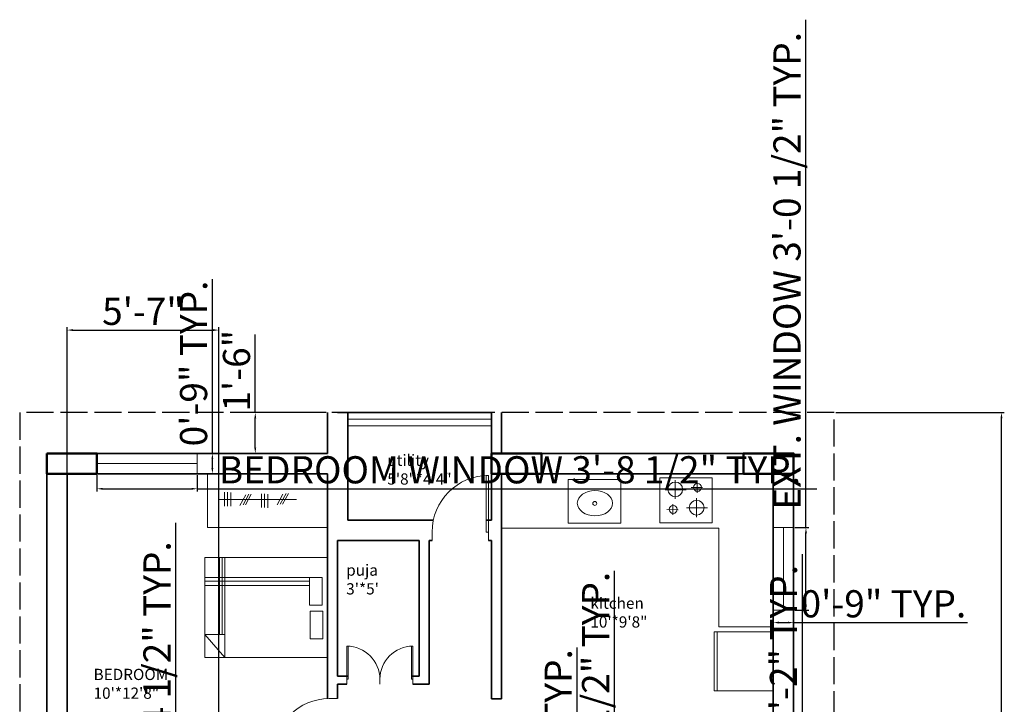
# Model space of a CAD drawing. Units: inches. Extents: x 2147 to 2722, y 2048 to 2905.
# Tile 3 of 3: x 2209 to 2644, y 2602 to 2905. Entities that reach past the tile are written whole.
import ezdxf

# ---------------------------------------------------------------- set-up
doc = ezdxf.new("R2010")
doc.units = ezdxf.units.IN
doc.linetypes.add('ACAD_ISO02W100', pattern=[15, 12, -3])
for name, color, linetype, lineweight in [('A-ANNO-DIMS', 2, 'Continuous', 18), ('A-AREA-IDEN', 7, 'Continuous', 18), ('A-COLS', 7, 'Continuous', 50), ('A-COLS-PATT', 252, 'Continuous', 13), ('A-DOOR', 3, 'Continuous', 18), ('A-EQPM', 9, 'Continuous', 18), ('A-FLOR-CASE', 8, 'Continuous', 18), ('A-FLOR-FIXT', 9, 'Continuous', 18), ('A-FURN', 8, 'Continuous', 18), ('A-GLAZ', 4, 'Continuous', 18), ('A-WALL', 7, 'Continuous', 35), ('C-PROP', 6, 'ACAD_ISO02W100', 25)]:
    doc.layers.add(name, color=color, linetype=linetype, lineweight=lineweight)
doc.styles.get("Standard").update_dxf_attribs({"font": 'arial.ttf'})
doc.dimstyles.new('ISO-25', dxfattribs={"dimtxt": 12, "dimasz": 2.5, "dimexe": 1.25, "dimexo": 0.625, "dimtad": 1, "dimdec": 0, "dimlunit": 4, "dimtxsty": 'Standard', "dimcen": 2.5, "dimadec": 0, "dimazin": 0, "dimtfac": 1, "dimtdec": 0, "dimtmove": 0, "dimatfit": 3, "dimfxl": 1, "dimarcsym": 0})

# ---------------------------------------------------------------- blocks, each defined once
blk = doc.blocks.new('*D1')
at = {"layer": 'A-ANNO-DIMS', "color": 0, "lineweight": -2, "transparency": 16777216}
for p, q in [((2569.22, 2730.99), (2643.73, 2730.99)), ((2642.48, 2133.49), (2642.48, 2728.49)), ((2569.22, 2130.99), (2643.73, 2130.99))]:
    blk.add_line(p, q, dxfattribs=at)
at = {"layer": 'A-ANNO-DIMS', "color": 0, "lineweight": 100, "transparency": 16777216}
for points in [[(2642.06, 2728.49), (2642.9, 2728.49), (2642.48, 2730.99)], [(2642.06, 2133.49), (2642.9, 2133.49), (2642.48, 2130.99)]]:
    blk.add_solid(points, dxfattribs=at)
at = {"layer": 'Defpoints', "color": 0, "lineweight": 100, "transparency": 16777216}
for p in [(2568.6, 2730.99), (2642.48, 2730.99), (2568.6, 2130.99)]:
    blk.add_point(p, dxfattribs=at)
at = {"layer": 'A-ANNO-DIMS', "color": 0, "transparency": 16777216, "insert": (2635.73, 2430.99), "char_height": 12, "attachment_point": 5, "rotation": 90}
blk.add_mtext("50'", dxfattribs=at)
blk = doc.blocks.new('*U3')
for p, q in [((0, 0), (0, -6)), ((40, 0), (40, -6))]:
    blk.add_line(p, q)
blk.add_lwpolyline([(0, 0), (0, 40), (1.75, 40), (1.75, 0)], close=True)
blk.add_arc((0, 0), 40, 0, 90)
blk = doc.blocks.new('*D7')
at = {"layer": 'A-ANNO-DIMS', "color": 0, "lineweight": -2, "transparency": 16777216}
for p, q in [((2312.71, 2730.99), (2312.71, 2765.51)), ((2343.97, 2730.99), (2311.46, 2730.99)), ((2312.71, 2715.49), (2312.71, 2728.49)), ((2343.97, 2712.99), (2311.46, 2712.99))]:
    blk.add_line(p, q, dxfattribs=at)
at = {"layer": 'A-ANNO-DIMS', "color": 0, "lineweight": 100, "transparency": 16777216}
for points in [[(2312.29, 2728.49), (2313.13, 2728.49), (2312.71, 2730.99)], [(2312.29, 2715.49), (2313.13, 2715.49), (2312.71, 2712.99)]]:
    blk.add_solid(points, dxfattribs=at)
at = {"layer": 'Defpoints', "color": 0, "lineweight": 100, "transparency": 16777216}
for p in [(2312.71, 2730.99), (2344.59, 2730.99), (2344.59, 2712.99)]:
    blk.add_point(p, dxfattribs=at)
at = {"layer": 'A-ANNO-DIMS', "color": 0, "transparency": 16777216, "insert": (2305.96, 2749.5), "char_height": 12, "attachment_point": 5, "rotation": 90}
blk.add_mtext('1\'-6"', dxfattribs=at)
blk = doc.blocks.new('BED-TWIN-PILLOW')
for p, q in [((6.6, 10.17), (6.6, 44.18)), ((7.66, 10.17), (7.66, 44.18)), ((8.88, 10.17), (8.88, 44.18)), ((46.28, 35.34), (0, 35.34)), ((46.28, 33.66), (0, 33.66)), ((46.28, 31.83), (0, 31.83)), ((8.88, 0), (0, 10.17))]:
    blk.add_line(p, q)
for points in [[(54.22, 44.18), (0, 44.18), (0, 0), (54.22, 0)], [(51.93, 35.34), (46.28, 35.34), (46.28, 23.14), (51.93, 23.14)], [(52.24, 20.39), (46.59, 20.39), (46.59, 8.19), (52.24, 8.19)], [(0, 0), (8.88, 0), (8.88, 10.17), (0, 10.17)]]:
    blk.add_lwpolyline(points, close=True)
blk = doc.blocks.new('WARDROBE')
for p, q in [((7.59, 9.5), (7.59, 15.59)), ((8.92, 9.5), (8.92, 15.59)), ((10.35, 9.4), (10.35, 15.5)), ((14.36, 9.78), (16.93, 14.55)), ((15.74, 10.07), (18.32, 14.83)), ((16.79, 10.07), (19.36, 14.83)), ((23.89, 8.83), (23.89, 14.93)), ((25.23, 8.83), (25.23, 14.93)), ((26.66, 8.73), (26.66, 14.83)), ((30.8, 10.05), (33.37, 14.82)), ((32.18, 10.34), (34.76, 15.1)), ((33.23, 10.34), (35.81, 15.1)), ((5.01, 12.45), (39.39, 12.45))]:
    blk.add_line(p, q)
blk.add_lwpolyline([(53.03, 23.8), (0, 23.8), (0, 0), (53.03, 0)], close=True)
blk = doc.blocks.new('WINDOW-BEDROOM')
blk.add_line((0, 4.5), (44.35, 4.5))
blk.add_lwpolyline([(0, 9), (44.35, 9), (44.35, 0), (0, 0)], close=True)
blk = doc.blocks.new('WINDOW-EXTERIOR')
blk.add_line((4.5, 36.51), (4.5, 0))
blk.add_lwpolyline([(0, 36.51), (9, 36.51), (9, 0), (0, 0)], close=True)
blk = doc.blocks.new('*D25')
at = {"layer": 'A-ANNO-DIMS', "color": 0, "lineweight": -2, "transparency": 16777216}
for p, q in [((2471.49, 2556.24), (2471.49, 2661.1)), ((2470.57, 2556.24), (2472.74, 2556.24)), ((2471.49, 2549.26), (2471.49, 2553.74)), ((2470.57, 2546.76), (2472.74, 2546.76))]:
    blk.add_line(p, q, dxfattribs=at)
at = {"layer": 'A-ANNO-DIMS', "color": 0, "lineweight": 100, "transparency": 16777216}
for points in [[(2471.08, 2553.74), (2471.91, 2553.74), (2471.49, 2556.24)], [(2471.08, 2549.26), (2471.91, 2549.26), (2471.49, 2546.76)]]:
    blk.add_solid(points, dxfattribs=at)
at = {"layer": 'Defpoints', "color": 0, "lineweight": 100, "transparency": 16777216}
for p in [(2469.94, 2556.24), (2471.49, 2556.24), (2469.94, 2546.76)]:
    blk.add_point(p, dxfattribs=at)
at = {"layer": 'A-ANNO-DIMS', "color": 0, "transparency": 16777216, "insert": (2464.66, 2609.92), "char_height": 12, "attachment_point": 5, "rotation": 90}
blk.add_mtext('0\'-9 1/2" TYP.', dxfattribs=at)
blk = doc.blocks.new('*D32')
at = {"layer": 'A-ANNO-DIMS', "color": 0, "lineweight": -2, "transparency": 16777216}
for p, q in [((2556.07, 2680.2), (2556.07, 2904.56)), ((2551.22, 2680.2), (2557.32, 2680.2)), ((2556.07, 2646.2), (2556.07, 2677.7)), ((2551.22, 2643.7), (2557.32, 2643.7))]:
    blk.add_line(p, q, dxfattribs=at)
at = {"layer": 'A-ANNO-DIMS', "color": 0, "lineweight": 100, "transparency": 16777216}
for points in [[(2555.66, 2677.7), (2556.49, 2677.7), (2556.07, 2680.2)], [(2555.66, 2646.2), (2556.49, 2646.2), (2556.07, 2643.7)]]:
    blk.add_solid(points, dxfattribs=at)
at = {"layer": 'Defpoints', "color": 0, "lineweight": 100, "transparency": 16777216}
for p in [(2550.6, 2680.2), (2556.07, 2680.2), (2550.6, 2643.7)]:
    blk.add_point(p, dxfattribs=at)
at = {"layer": 'A-ANNO-DIMS', "color": 0, "transparency": 16777216, "insert": (2549.24, 2793.63), "char_height": 12, "attachment_point": 5, "rotation": 90}
blk.add_mtext('EXT. WINDOW 3\'-0 1/2" TYP.', dxfattribs=at)
blk = doc.blocks.new('*D33')
at = {"layer": 'A-ANNO-DIMS', "color": 0, "lineweight": -2, "transparency": 16777216}
for p, q in [((2541.6, 2643.07), (2541.6, 2636.97)), ((2550.6, 2643.07), (2550.6, 2636.97)), ((2544.1, 2638.22), (2548.1, 2638.22)), ((2550.6, 2638.22), (2627.49, 2638.22))]:
    blk.add_line(p, q, dxfattribs=at)
at = {"layer": 'A-ANNO-DIMS', "color": 0, "lineweight": 100, "transparency": 16777216}
for points in [[(2544.1, 2638.64), (2544.1, 2637.81), (2541.6, 2638.22)], [(2548.1, 2638.64), (2548.1, 2637.81), (2550.6, 2638.22)]]:
    blk.add_solid(points, dxfattribs=at)
at = {"layer": 'Defpoints', "color": 0, "lineweight": 100, "transparency": 16777216}
for p in [(2541.6, 2643.7), (2550.6, 2643.7), (2550.6, 2638.22)]:
    blk.add_point(p, dxfattribs=at)
at = {"layer": 'A-ANNO-DIMS', "color": 0, "transparency": 16777216, "insert": (2590.3, 2644.97), "char_height": 12, "attachment_point": 5}
blk.add_mtext('0\'-9" TYP.', dxfattribs=at)
blk = doc.blocks.new('*D37')
at = {"layer": 'A-ANNO-DIMS', "color": 0, "lineweight": -2, "transparency": 16777216}
for p, q in [((2454.9, 2540.96), (2454.9, 2627.18)), ((2453.83, 2540.96), (2456.15, 2540.96)), ((2454.9, 2532.23), (2454.9, 2538.46)), ((2453.83, 2529.73), (2456.15, 2529.73))]:
    blk.add_line(p, q, dxfattribs=at)
at = {"layer": 'A-ANNO-DIMS', "color": 0, "lineweight": 100, "transparency": 16777216}
for points in [[(2454.48, 2538.46), (2455.32, 2538.46), (2454.9, 2540.96)], [(2454.48, 2532.23), (2455.32, 2532.23), (2454.9, 2529.73)]]:
    blk.add_solid(points, dxfattribs=at)
at = {"layer": 'Defpoints', "color": 0, "lineweight": 100, "transparency": 16777216}
for p in [(2453.21, 2540.96), (2454.9, 2540.96), (2453.21, 2529.73)]:
    blk.add_point(p, dxfattribs=at)
at = {"layer": 'A-ANNO-DIMS', "color": 0, "transparency": 16777216, "insert": (2448.15, 2585.32), "char_height": 12, "attachment_point": 5, "rotation": 90}
blk.add_mtext('0\'-11" TYP.', dxfattribs=at)
blk = doc.blocks.new('*D40')
at = {"layer": 'A-ANNO-DIMS', "color": 0, "lineweight": -2, "transparency": 16777216}
for p, q in [((2242.74, 2703.36), (2242.74, 2696.09)), ((2287.1, 2703.36), (2287.1, 2696.09)), ((2245.24, 2697.34), (2284.6, 2697.34)), ((2287.1, 2697.34), (2560.91, 2697.34))]:
    blk.add_line(p, q, dxfattribs=at)
at = {"layer": 'A-ANNO-DIMS', "color": 0, "lineweight": 100, "transparency": 16777216}
for points in [[(2245.24, 2697.75), (2245.24, 2696.92), (2242.74, 2697.34)], [(2284.6, 2697.75), (2284.6, 2696.92), (2287.1, 2697.34)]]:
    blk.add_solid(points, dxfattribs=at)
at = {"layer": 'Defpoints', "color": 0, "lineweight": 100, "transparency": 16777216}
for p in [(2242.74, 2703.99), (2287.1, 2703.99), (2287.1, 2697.34)]:
    blk.add_point(p, dxfattribs=at)
at = {"layer": 'A-ANNO-DIMS', "color": 0, "transparency": 16777216, "insert": (2425.25, 2704.17), "char_height": 12, "attachment_point": 5}
blk.add_mtext('BEDROOM WINDOW 3\'-8 1/2" TYP.', dxfattribs=at)
blk = doc.blocks.new('*D41')
at = {"layer": 'A-ANNO-DIMS', "color": 0, "lineweight": -2, "transparency": 16777216}
for p, q in [((2293.75, 2712.99), (2293.75, 2789.89)), ((2287.72, 2712.99), (2295, 2712.99)), ((2293.75, 2706.49), (2293.75, 2710.49)), ((2287.72, 2703.99), (2295, 2703.99))]:
    blk.add_line(p, q, dxfattribs=at)
at = {"layer": 'A-ANNO-DIMS', "color": 0, "lineweight": 100, "transparency": 16777216}
for points in [[(2293.33, 2710.49), (2294.16, 2710.49), (2293.75, 2712.99)], [(2293.33, 2706.49), (2294.16, 2706.49), (2293.75, 2703.99)]]:
    blk.add_solid(points, dxfattribs=at)
at = {"layer": 'Defpoints', "color": 0, "lineweight": 100, "transparency": 16777216}
for p in [(2287.1, 2712.99), (2293.75, 2712.99), (2287.1, 2703.99)]:
    blk.add_point(p, dxfattribs=at)
at = {"layer": 'A-ANNO-DIMS', "color": 0, "transparency": 16777216, "insert": (2287, 2752.69), "char_height": 12, "attachment_point": 5, "rotation": 90}
blk.add_mtext('0\'-9" TYP.', dxfattribs=at)
blk = doc.blocks.new('*D42')
at = {"layer": 'A-ANNO-DIMS', "color": 0, "lineweight": -2, "transparency": 16777216}
for p, q in [((2554.51, 2464.55), (2554.51, 2668.49)), ((2551.22, 2464.55), (2555.76, 2464.55)), ((2554.51, 2440.93), (2554.51, 2462.05)), ((2551.22, 2438.43), (2555.76, 2438.43))]:
    blk.add_line(p, q, dxfattribs=at)
at = {"layer": 'A-ANNO-DIMS', "color": 0, "lineweight": 100, "transparency": 16777216}
for points in [[(2554.1, 2462.05), (2554.93, 2462.05), (2554.51, 2464.55)], [(2554.1, 2440.93), (2554.93, 2440.93), (2554.51, 2438.43)]]:
    blk.add_solid(points, dxfattribs=at)
at = {"layer": 'Defpoints', "color": 0, "lineweight": 100, "transparency": 16777216}
for p in [(2550.6, 2464.55), (2554.51, 2464.55), (2550.6, 2438.43)]:
    blk.add_point(p, dxfattribs=at)
at = {"layer": 'A-ANNO-DIMS', "color": 0, "transparency": 16777216, "insert": (2547.68, 2567.77), "char_height": 12, "attachment_point": 5, "rotation": 90}
blk.add_mtext('BATH WINDOW 2\'-2" TYP.', dxfattribs=at)
blk = doc.blocks.new('*D44')
at = {"layer": 'A-ANNO-DIMS', "color": 0, "lineweight": -2, "transparency": 16777216}
for p, q in [((2277.67, 2415.1), (2277.67, 2682.36)), ((2272.22, 2415.1), (2278.92, 2415.1)), ((2277.67, 2377.15), (2277.67, 2412.6)), ((2272.22, 2374.65), (2278.92, 2374.65))]:
    blk.add_line(p, q, dxfattribs=at)
at = {"layer": 'A-ANNO-DIMS', "color": 0, "lineweight": 100, "transparency": 16777216}
for points in [[(2277.25, 2412.6), (2278.08, 2412.6), (2277.67, 2415.1)], [(2277.25, 2377.15), (2278.08, 2377.15), (2277.67, 2374.65)]]:
    blk.add_solid(points, dxfattribs=at)
at = {"layer": 'Defpoints', "color": 0, "lineweight": 100, "transparency": 16777216}
for p in [(2271.6, 2415.1), (2277.67, 2415.1), (2271.6, 2374.65)]:
    blk.add_point(p, dxfattribs=at)
at = {"layer": 'A-ANNO-DIMS', "color": 0, "transparency": 16777216, "insert": (2270.83, 2549.98), "char_height": 12, "attachment_point": 5, "rotation": 90}
blk.add_mtext('PASSAGE WINDOW 3\'-4 1/2" TYP.', dxfattribs=at)
blk = doc.blocks.new('*D48')
at = {"layer": 'A-ANNO-DIMS', "color": 0, "lineweight": -2, "transparency": 16777216}
for p, q in [((2229.6, 2266.77), (2229.6, 2768.69)), ((2296.59, 2266.77), (2296.59, 2768.69)), ((2232.1, 2767.44), (2294.09, 2767.44))]:
    blk.add_line(p, q, dxfattribs=at)
at = {"layer": 'A-ANNO-DIMS', "color": 0, "lineweight": 100, "transparency": 16777216}
for points in [[(2232.1, 2767.86), (2232.1, 2767.02), (2229.6, 2767.44)], [(2294.09, 2767.86), (2294.09, 2767.02), (2296.59, 2767.44)]]:
    blk.add_solid(points, dxfattribs=at)
at = {"layer": 'Defpoints', "color": 0, "lineweight": 100, "transparency": 16777216}
for p in [(2296.59, 2767.44), (2229.6, 2266.14), (2296.59, 2266.14)]:
    blk.add_point(p, dxfattribs=at)
at = {"layer": 'A-ANNO-DIMS', "color": 0, "transparency": 16777216, "insert": (2263.1, 2774.17), "char_height": 12, "attachment_point": 5}
blk.add_mtext('5\'-7"', dxfattribs=at)

msp = doc.modelspace()

# ---------------------------------------------------------------- hatches: boundary and pattern name
at = {"layer": 'A-COLS-PATT'}
h = msp.add_hatch(dxfattribs=at)
h.set_pattern_fill('AR-SAND', color=256, scale=50)
h.paths.add_polyline_path([(2242.74, 2712.99), (2220.6, 2712.99), (2220.6, 2703.99), (2242.74, 2703.99)])
h = msp.add_hatch(dxfattribs=at)
h.set_pattern_fill('AR-SAND', color=256, scale=5)
h.paths.add_polyline_path([(2439.24, 2712.96), (2417.09, 2712.96), (2417.09, 2703.96), (2421.59, 2703.96), (2421.59, 2703.99), (2439.24, 2703.99)])
h.paths.add_polyline_path([(2550.6, 2712.99), (2528.45, 2712.99), (2528.45, 2703.99), (2541.27, 2703.99), (2550.6, 2703.99)])
h.paths.add_polyline_path([(2229.6, 2593.61), (2220.6, 2593.61), (2220.6, 2571.86), (2229.6, 2571.86), (2229.6, 2574.49), (2230.08, 2574.49), (2230.08, 2578.99), (2229.6, 2578.99)])
h.paths.add_polyline_path([(2229.6, 2152.74), (2220.6, 2152.74), (2220.6, 2130.99), (2229.6, 2130.99), (2230.08, 2130.99), (2230.08, 2139.99), (2229.6, 2139.99)])
h.paths.add_polyline_path([(2301.09, 2152.74), (2296.59, 2152.74), (2296.59, 2140.02), (2301.09, 2140.03)])
h.paths.add_polyline_path([(2306.03, 2152.74), (2301.09, 2152.74), (2301.09, 2140.03), (2306.03, 2140.03)])
h.paths.add_polyline_path([(2306.03, 2140.03), (2296.55, 2140.02), (2296.55, 2130.99), (2306.03, 2130.99)])
h.paths.add_polyline_path([(2426.67, 2152.74), (2421.59, 2152.74), (2421.59, 2140.08), (2426.67, 2140.08)])
h.paths.add_polyline_path([(2421.59, 2152.74), (2417.19, 2152.74), (2417.19, 2140.08), (2421.59, 2140.08)])
h.paths.add_polyline_path([(2426.67, 2140.08), (2421.59, 2140.08), (2417.19, 2140.08), (2417.19, 2130.99), (2426.67, 2130.99)])

# ---------------------------------------------------------------- linework, layer by layer
at = {"layer": 'A-COLS'}
for points in [[(2220.6, 2712.99), (2242.74, 2712.99), (2242.74, 2703.99), (2220.6, 2703.99)], [(2417.09, 2712.96), (2439.24, 2712.96), (2439.24, 2703.96), (2417.09, 2703.96)]]:
    msp.add_lwpolyline(points, close=True, dxfattribs=at)
msp.add_lwpolyline([(2541.27, 2703.99), (2528.45, 2703.99), (2528.45, 2712.99), (2550.6, 2712.99), (2550.6, 2703.99), (2541.27, 2703.99)], dxfattribs=at)
at = {"layer": 'A-EQPM'}
for p, q in [((2498.33, 2701.19), (2498.33, 2692.88)), ((2505.37, 2697.96), (2510.39, 2697.84)), ((2508.03, 2695.6), (2508.03, 2700.22)), ((2493.86, 2696.94), (2503.08, 2696.94)), ((2497.26, 2685.86), (2497.26, 2690.48)), ((2507.77, 2693.14), (2507.77, 2684.83)), ((2494.6, 2688.22), (2499.61, 2688.1)), ((2503.29, 2688.9), (2512.51, 2688.9)), ((2515.48, 2608.13), (2515.48, 2634.16)), ((2515.48, 2634.16), (2541.59, 2634.16)), ((2516.85, 2608.13), (2516.85, 2634.16)), ((2541.59, 2608.13), (2515.48, 2608.13))]:
    msp.add_line(p, q, dxfattribs=at)
msp.add_lwpolyline([(2514.62, 2682.29), (2491.47, 2682.29), (2491.47, 2702.17), (2514.62, 2702.17)], close=True, dxfattribs=at)
for centre, radius in [((2498.32, 2697.05), 3.26), ((2508.15, 2697.96), 1.74), ((2497.38, 2688.22), 1.74), ((2507.76, 2689.01), 3.26)]:
    msp.add_circle(centre, radius, dxfattribs=at)
at = {"layer": 'A-FLOR-CASE'}
for p, q in [((2421.59, 2703.96), (2421.59, 2679.96)), ((2421.59, 2679.96), (2517.59, 2679.96)), ((2517.59, 2636.3), (2517.59, 2679.96)), ((2541.59, 2636.3), (2517.59, 2636.3))]:
    msp.add_line(p, q, dxfattribs=at)
at = {"layer": 'A-FLOR-FIXT'}
msp.add_lwpolyline([(2450.94, 2682.13), (2474.21, 2682.13), (2474.21, 2701.38), (2450.94, 2701.38)], close=True, dxfattribs=at)
msp.add_circle((2462.74, 2690.88), 0.868, dxfattribs=at)
msp.add_ellipse((2462.84, 2690.98), major_axis=(7.81, 0), ratio=0.71581, dxfattribs=at)
at = {"layer": 'A-GLAZ'}
msp.add_line((2353.59, 2728.06), (2417.09, 2728.06), dxfattribs=at)
msp.add_lwpolyline([(2353.59, 2730.99), (2417.09, 2730.99), (2417.09, 2725.13), (2353.59, 2725.13)], close=True, dxfattribs=at)
at = {"layer": 'A-WALL'}
for p, q in [((2344.59, 2730.99), (2344.59, 2712.99)), ((2344.59, 2730.99), (2344.59, 2712.99)), ((2417.09, 2730.99), (2349.09, 2730.99)), ((2353.59, 2730.99), (2353.59, 2683.49)), ((2417.09, 2725.13), (2417.09, 2730.99)), ((2421.59, 2720.63), (2421.59, 2730.99)), ((2417.09, 2725.13), (2417.09, 2683.49)), ((2421.59, 2720.63), (2421.59, 2712.99)), ((2220.6, 2130.99), (2220.6, 2712.99)), ((2220.6, 2712.99), (2220.6, 2578.99)), ((2229.6, 2712.99), (2220.6, 2712.99)), ((2344.59, 2712.99), (2229.6, 2712.99)), ((2421.59, 2712.99), (2541.6, 2712.99)), ((2541.6, 2712.99), (2550.6, 2712.99)), ((2550.6, 2131.13), (2550.6, 2712.99)), ((2229.6, 2703.99), (2229.6, 2578.99)), ((2344.59, 2703.99), (2229.6, 2703.99)), ((2344.59, 2703.99), (2344.59, 2674.49)), ((2421.59, 2703.99), (2541.6, 2703.99)), ((2421.59, 2703.99), (2421.59, 2604.63)), ((2541.59, 2604.13), (2541.6, 2703.99)), ((2353.59, 2683.49), (2391.41, 2683.49)), ((2414.72, 2683.49), (2417.09, 2683.49)), ((2344.59, 2674.49), (2344.59, 2604.66)), ((2349.09, 2674.49), (2385.09, 2674.49)), ((2349.09, 2674.49), (2349.09, 2614.49)), ((2349.09, 2674.49), (2385.09, 2674.49)), ((2385.09, 2674.49), (2385.09, 2614.49)), ((2389.59, 2674.49), (2389.59, 2610.99)), ((2389.59, 2674.49), (2390.85, 2674.49)), ((2390.85, 2674.49), (2389.59, 2674.49)), ((2417.09, 2674.49), (2415.82, 2674.49)), ((2415.82, 2674.49), (2417.09, 2674.49)), ((2417.09, 2674.49), (2417.09, 2604.63)), ((2353.77, 2614.49), (2349.09, 2614.49)), ((2349.09, 2610.99), (2349.09, 2604.67)), ((2353.13, 2610.99), (2349.09, 2610.99)), ((2367.82, 2614.49), (2367.71, 2614.49)), ((2385.09, 2614.49), (2381.76, 2614.49)), ((2389.59, 2610.99), (2382.4, 2610.99)), ((2417.09, 2604.63), (2417.09, 2604.59)), ((2417.09, 2604.59), (2421.59, 2604.57)), ((2421.59, 2604.63), (2421.59, 2604.57)), ((2541.59, 2604.63), (2541.59, 2580.48))]:
    msp.add_line(p, q, dxfattribs=at)
at = {"layer": 'C-PROP'}
msp.add_line((2208.6, 2730.99), (2208.6, 2582.9), dxfattribs=at)
msp.add_lwpolyline([(2208.6, 2130.99), (2568.6, 2130.99), (2568.6, 2730.99), (2208.6, 2730.99)], close=True, dxfattribs=at)

# ---------------------------------------------------------------- block references
at = {"layer": 'A-DOOR'}
for p, xscale, yscale, zscale in [((2415.82, 2678.24), -0.6242076431293141, 0.6242076431293141, 0.6242076431293141), ((2353.13, 2613.19), 0.3659458524126017, 0.3659458524126017, 0.3659458524126017), ((2382.4, 2613.19), -0.3659458524126017, 0.3659458524126017, 0.3659458524126017)]:
    msp.add_blockref('*U3', p, dxfattribs=dict(at, xscale=xscale, yscale=yscale, zscale=zscale))
at = {"layer": 'A-DOOR', "xscale": 0.6127871622533858, "yscale": 0.6127871622533858, "zscale": 0.6127871622533858, "rotation": 90.00000000000003}
msp.add_blockref('*U3', (2345.42, 2580.16), dxfattribs=at)
at = {"layer": 'A-FLOR-CASE'}
msp.add_blockref('WARDROBE', (2291.57, 2680.19), dxfattribs=at)
at = {"layer": 'A-FURN'}
msp.add_blockref('BED-TWIN-PILLOW', (2290.37, 2622.82), dxfattribs=at)
at = {"layer": 'A-GLAZ'}
for name, p in [('WINDOW-BEDROOM', (2242.74, 2703.99)), ('WINDOW-EXTERIOR', (2541.6, 2643.7))]:
    msp.add_blockref(name, p, dxfattribs=at)

# ---------------------------------------------------------------- texts
at = {"layer": 'A-AREA-IDEN', "char_height": 4.968, "attachment_point": 1}
for s, insert in [('utility\\P5\'8"*4\'4"', (2371.07, 2712.43)), ("puja\\P3'*5'", (2352.9, 2663.9)), ('kitchen\\P10\'*9\'8"', (2460.8, 2649.28)), ('BEDROOM\\P10\'*12\'8"', (2241.25, 2617.81))]:
    msp.add_mtext_dynamic_manual_height_columns(s, width=78.277, gutter_width=24.84, heights=[0], dxfattribs=dict(at, insert=insert))

# ---------------------------------------------------------------- dimensions: what is measured, and where the dimension line sits
at = {"layer": 'A-ANNO-DIMS'}
for base, p1, p2, text, picture, middle in [((2556.07, 2680.2), (2550.6, 2643.7), (2550.6, 2680.2), 'EXT. WINDOW <> TYP.', '*D32', (2549.24, 2793.63)), ((2293.75, 2712.99), (2287.1, 2703.99), (2287.1, 2712.99), '<> TYP.', '*D41', (2287, 2752.69)), ((2277.6651, 2415.1016), (2271.597, 2374.6474), (2271.597, 2415.1016), 'PASSAGE WINDOW <> TYP.', '*D44', (2270.8273, 2549.981)), ((2554.51, 2464.55), (2550.6, 2438.43), (2550.6, 2464.55), 'BATH WINDOW <> TYP.', '*D42', (2547.68, 2567.77)), ((2471.49, 2556.24), (2469.94, 2546.76), (2469.94, 2556.24), '<> TYP.', '*D25', (2464.66, 2609.92)), ((2454.9, 2540.96), (2453.21, 2529.73), (2453.21, 2540.96), '<> TYP.', '*D37', (2448.15, 2585.32))]:
    dim = msp.add_linear_dim(base=base, p1=p1, p2=p2, angle=90, text=text, dimstyle='ISO-25', override={"dimdec": 1, "dimlfac": 1, "dimrnd": 0, "dimzin": 1, "dimdsep": 46, "dimlunit": 4, "dimfrac": 2}, dxfattribs=at)
    dim.commit()
    dim.dimension.update_dxf_attribs({"geometry": picture, "text_midpoint": middle})
dim = msp.add_linear_dim(base=(2296.59, 2767.44), p1=(2229.6, 2266.14), p2=(2296.59, 2266.14), dimstyle='ISO-25', override={"dimdec": 1, "dimlfac": 1, "dimrnd": 0, "dimzin": 1, "dimdsep": 46, "dimlunit": 4, "dimfrac": 2}, dxfattribs=at)
dim.commit()
dim.dimension.update_dxf_attribs({"geometry": '*D48', "text_midpoint": (2263.1, 2774.17)})
for base, p1, p2, picture, middle in [((2312.71, 2730.99), (2344.59, 2712.99), (2344.59, 2730.99), '*D7', (2305.96, 2749.5)), ((2642.48, 2730.99), (2568.6, 2130.99), (2568.6, 2730.99), '*D1', (2635.73, 2430.99))]:
    dim = msp.add_linear_dim(base=base, p1=p1, p2=p2, angle=90, dimstyle='ISO-25', override={"dimclrd": 0, "dimclre": 0, "dimclrt": 0}, dxfattribs=at)
    dim.commit()
    dim.dimension.update_dxf_attribs({"geometry": picture, "text_midpoint": middle})
for base, p1, p2, text, picture, middle in [((2287.1, 2697.34), (2242.74, 2703.99), (2287.1, 2703.99), 'BEDROOM WINDOW <> TYP.', '*D40', (2425.25, 2704.17)), ((2550.6, 2638.22), (2541.6, 2643.7), (2550.6, 2643.7), '<> TYP.', '*D33', (2590.3, 2644.97))]:
    dim = msp.add_linear_dim(base=base, p1=p1, p2=p2, text=text, dimstyle='ISO-25', override={"dimdec": 1, "dimlfac": 1, "dimrnd": 0, "dimzin": 1, "dimdsep": 46, "dimlunit": 4, "dimfrac": 2}, dxfattribs=at)
    dim.commit()
    dim.dimension.update_dxf_attribs({"geometry": picture, "text_midpoint": middle})

doc.saveas('drawing.dxf')
